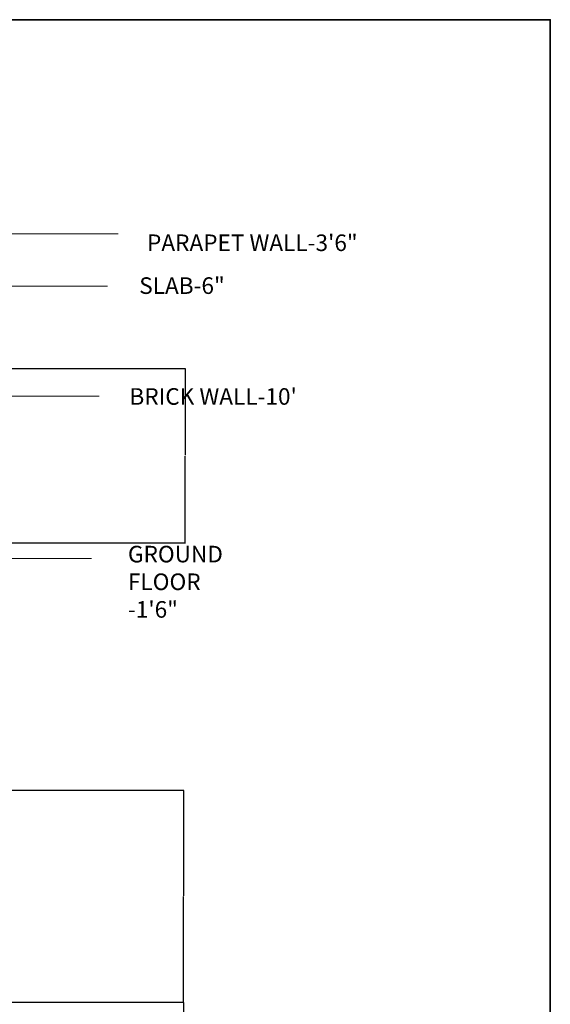
# Model space of a CAD drawing. Units: inches. Extents: x 2250 to 3547, y 1387 to 2604.
# Tile 11 of 11: x 3291 to 3547, y 2129 to 2604. Entities that reach past the tile are written whole.
import ezdxf

# ---------------------------------------------------------------- set-up
doc = ezdxf.new("R2010")
doc.units = ezdxf.units.IN
for name, color, linetype, lineweight in [('A-ANNO-DIMS', 2, 'Continuous', 18), ('A-ANNO-TEXT', 7, 'Continuous', 18), ('A-ANNO-TTLB', 7, 'Continuous', 35)]:
    doc.layers.add(name, color=color, linetype=linetype, lineweight=lineweight)
doc.styles.get("Standard").update_dxf_attribs({"font": 'arial.ttf'})
doc.dimstyles.get("Standard").update_dxf_attribs({"dimtxt": 0.18, "dimasz": 0.18, "dimexe": 0.18, "dimexo": 0.0625, "dimgap": 0.09, "dimtad": 0, "dimtih": 1, "dimtoh": 1, "dimdec": 4, "dimzin": 0, "dimdsep": 46, "dimtxsty": 'Standard', "dimcen": 0.09, "dimadec": 0, "dimazin": 0, "dimtfac": 1, "dimtdec": 4, "dimtofl": 0, "dimtmove": 0, "dimatfit": 3, "dimfxl": 1, "dimtolj": 1, "dimtzin": 0, "dimarcsym": 0})

# ---------------------------------------------------------------- blocks, each defined once
blk = doc.blocks.new('*D90')
at = {"layer": 'A-ANNO-DIMS', "color": 0, "lineweight": -2, "transparency": 16777216}
for p, q in [((3283.69, 2130.34), (3370.22, 2130.34)), ((3370.04, 2130.16), (3370.04, 2093.38)), ((3370.04, 2056.23), (3370.04, 2093.01)), ((3283.69, 2056.05), (3370.22, 2056.05))]:
    blk.add_line(p, q, dxfattribs=at)
at = {"layer": 'A-ANNO-DIMS', "color": 0, "transparency": 16777216}
for points in [[(3370.01, 2130.16), (3370.07, 2130.16), (3370.04, 2130.34)], [(3370.01, 2056.23), (3370.07, 2056.23), (3370.04, 2056.05)]]:
    blk.add_solid(points, dxfattribs=at)
at = {"layer": 'Defpoints', "color": 0, "transparency": 16777216}
for p in [(3283.63, 2130.34), (3370.04, 2130.34), (3283.63, 2056.05)]:
    blk.add_point(p, dxfattribs=at)
at = {"layer": 'A-ANNO-DIMS', "color": 0, "transparency": 16777216, "insert": (3370.04, 2093.2), "char_height": 0.18, "attachment_point": 5}
blk.add_mtext('\\A1;74.29', dxfattribs=at)
blk = doc.blocks.new('*D91')
at = {"layer": 'A-ANNO-DIMS', "color": 0, "lineweight": -2, "transparency": 16777216}
for p, q in [((3283.69, 2232.56), (3370.22, 2232.56)), ((3370.04, 2232.38), (3370.04, 2181.63)), ((3370.04, 2130.52), (3370.04, 2181.27)), ((3283.69, 2130.34), (3370.22, 2130.34))]:
    blk.add_line(p, q, dxfattribs=at)
at = {"layer": 'A-ANNO-DIMS', "color": 0, "transparency": 16777216}
for points in [[(3370.01, 2232.38), (3370.07, 2232.38), (3370.04, 2232.56)], [(3370.01, 2130.52), (3370.07, 2130.52), (3370.04, 2130.34)]]:
    blk.add_solid(points, dxfattribs=at)
at = {"layer": 'Defpoints', "color": 0, "transparency": 16777216}
for p in [(3283.63, 2232.56), (3370.04, 2232.56), (3283.63, 2130.34)]:
    blk.add_point(p, dxfattribs=at)
at = {"layer": 'A-ANNO-DIMS', "color": 0, "transparency": 16777216, "insert": (3370.04, 2181.45), "char_height": 0.18, "attachment_point": 5}
blk.add_mtext('\\A1;102.22', dxfattribs=at)
blk = doc.blocks.new('*D113')
at = {"layer": 'A-ANNO-DIMS', "color": 0, "lineweight": -2, "transparency": 16777216}
for p, q in [((3048.42, 2435.95), (3371.04, 2435.95)), ((3370.86, 2435.77), (3370.86, 2394.13)), ((3370.86, 2352.13), (3370.86, 2393.77)), ((3048.42, 2351.95), (3371.04, 2351.95))]:
    blk.add_line(p, q, dxfattribs=at)
at = {"layer": 'A-ANNO-DIMS', "color": 0, "transparency": 16777216}
for points in [[(3370.83, 2435.77), (3370.89, 2435.77), (3370.86, 2435.95)], [(3370.83, 2352.13), (3370.89, 2352.13), (3370.86, 2351.95)]]:
    blk.add_solid(points, dxfattribs=at)
at = {"layer": 'Defpoints', "color": 0, "transparency": 16777216}
for p in [(3048.36, 2435.95), (3370.86, 2435.95), (3048.36, 2351.95)]:
    blk.add_point(p, dxfattribs=at)
at = {"layer": 'A-ANNO-DIMS', "color": 0, "transparency": 16777216, "insert": (3370.86, 2393.95), "char_height": 0.18, "attachment_point": 5}
blk.add_mtext('\\A1;84', dxfattribs=at)

msp = doc.modelspace()

# ---------------------------------------------------------------- linework, layer by layer
at = {"layer": 'A-ANNO-TEXT'}
for p, q in [((3283.6288, 2500.9984), (3338.5083, 2500.9984)), ((3281.9557, 2475.6362), (3333.3809, 2475.6362)), ((3283.6288, 2422.6027), (3329.2305, 2422.6027)), ((3276.8191, 2344.3195), (3325.6618, 2344.3195))]:
    msp.add_line(p, q, dxfattribs=at)
at = {"layer": 'A-ANNO-TTLB'}
msp.add_lwpolyline([(2250.1093, 2604.1988), (3546.995, 2604.1988), (3546.995, 1386.7251), (2250.1093, 1386.7251)], close=True, dxfattribs=at)

# ---------------------------------------------------------------- texts
at = {"layer": 'A-ANNO-TEXT', "char_height": 8, "attachment_point": 1}
for s, width, insert in [('PARAPET WALL-3\'6"', 116.733565, (3352.4094, 2500.6204)), ('SLAB-6"', 54.822246, (3348.6373, 2479.9404)), ("BRICK WALL-10'", 96.331423, (3343.9177, 2426.4865)), ('GROUND FLOOR -1\'6"', 61.605089, (3343.1911, 2350.452))]:
    msp.add_mtext_dynamic_manual_height_columns(s, width=width, gutter_width=12.5, heights=[0], dxfattribs=dict(at, insert=insert))

# ---------------------------------------------------------------- dimensions: what is measured, and where the dimension line sits
at = {"layer": 'A-ANNO-DIMS'}
for base, p1, p2, override, picture, middle in [((3370.8583, 2435.9493), (3048.3624, 2351.9493), (3048.3624, 2435.9493), {"dimdec": 0, "dimlfac": 1, "dimrnd": 0, "dimzin": 0, "dimdsep": 46, "dimlunit": 2}, '*D113', (3370.8583, 2393.9493)), ((3370.0441, 2232.5639), (3283.6288, 2130.3411), (3283.6288, 2232.5639), {"dimdec": 2, "dimlfac": 1, "dimrnd": 0, "dimzin": 0, "dimdsep": 46, "dimlunit": 2}, '*D91', (3370.0441, 2181.4525)), ((3370.0441, 2130.3411), (3283.6288, 2056.0503), (3283.6288, 2130.3411), {"dimdec": 2, "dimlfac": 1, "dimrnd": 0, "dimzin": 0, "dimdsep": 46, "dimlunit": 2}, '*D90', (3370.0441, 2093.1957))]:
    dim = msp.add_linear_dim(base=base, p1=p1, p2=p2, angle=90, dimstyle='Standard', override=override, dxfattribs=at)
    dim.commit()
    dim.dimension.update_dxf_attribs({"geometry": picture, "text_midpoint": middle})

doc.saveas('drawing.dxf')
